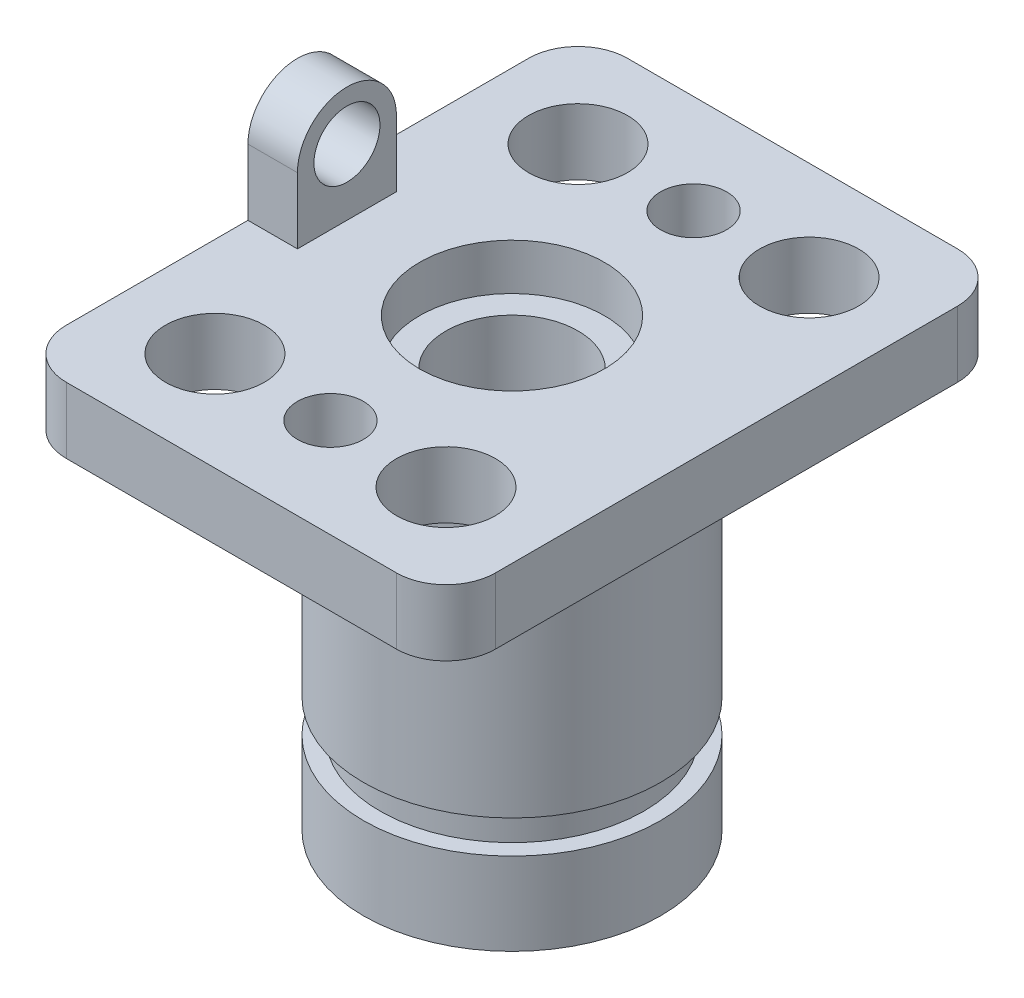
ISO-10303-21;
HEADER;
FILE_DESCRIPTION(('STEP AP214'),'2;1');
FILE_NAME('part.step','',(''),(''),'','','');
FILE_SCHEMA(('AUTOMOTIVE_DESIGN { 1 0 10303 214 1 1 1 1 }'));
ENDSEC;
DATA;
#1=APPLICATION_CONTEXT('core data for automotive mechanical design processes');
#2=APPLICATION_PROTOCOL_DEFINITION('international standard','automotive_design',2000,#1);
#3=PRODUCT_CONTEXT('',#1,'mechanical');
#4=PRODUCT('Part','Part','',(#3));
#5=PRODUCT_RELATED_PRODUCT_CATEGORY('part','',(#4));
#6=PRODUCT_DEFINITION_FORMATION('','',#4);
#7=PRODUCT_DEFINITION_CONTEXT('part definition',#1,'design');
#8=PRODUCT_DEFINITION('design','',#6,#7);
#9=PRODUCT_DEFINITION_SHAPE('','',#8);
#10=(LENGTH_UNIT() NAMED_UNIT(*) SI_UNIT(.MILLI.,.METRE.));
#11=(NAMED_UNIT(*) PLANE_ANGLE_UNIT() SI_UNIT($,.RADIAN.));
#12=(NAMED_UNIT(*) SI_UNIT($,.STERADIAN.) SOLID_ANGLE_UNIT());
#13=UNCERTAINTY_MEASURE_WITH_UNIT(LENGTH_MEASURE(1.E-05),#10,'distance_accuracy_value','');
#14=(GEOMETRIC_REPRESENTATION_CONTEXT(3) GLOBAL_UNCERTAINTY_ASSIGNED_CONTEXT((#13)) GLOBAL_UNIT_ASSIGNED_CONTEXT((#10,
#11,#12)) REPRESENTATION_CONTEXT('',''));
#15=CARTESIAN_POINT('',(0.,0.,0.));
#16=DIRECTION('',(0.,0.,1.));
#17=DIRECTION('',(1.,0.,0.));
#18=AXIS2_PLACEMENT_3D('',#15,#16,#17);
#19=CARTESIAN_POINT('',(0.,135.,0.));
#20=DIRECTION('',(0.,-1.,0.));
#21=DIRECTION('',(0.,0.,-1.));
#22=AXIS2_PLACEMENT_3D('',#19,#20,#21);
#23=PLANE('',#22);
#24=CARTESIAN_POINT('',(35.,135.,-55.));
#25=DIRECTION('',(0.,1.,0.));
#26=DIRECTION('',(0.,0.,1.));
#27=AXIS2_PLACEMENT_3D('',#24,#25,#26);
#28=CIRCLE('',#27,15.);
#29=CARTESIAN_POINT('',(35.,135.,-40.));
#30=VERTEX_POINT('',#29);
#31=EDGE_CURVE('E224',#30,#30,#28,.T.);
#32=ORIENTED_EDGE('',*,*,#31,.F.);
#33=EDGE_LOOP('',(#32));
#34=FACE_BOUND('',#33,.T.);
#35=CARTESIAN_POINT('',(0.,135.,-55.));
#36=DIRECTION('',(0.,1.,0.));
#37=DIRECTION('',(0.,0.,1.));
#38=AXIS2_PLACEMENT_3D('',#35,#36,#37);
#39=CIRCLE('',#38,10.);
#40=CARTESIAN_POINT('',(0.,135.,-45.));
#41=VERTEX_POINT('',#40);
#42=EDGE_CURVE('E226',#41,#41,#39,.T.);
#43=ORIENTED_EDGE('',*,*,#42,.F.);
#44=EDGE_LOOP('',(#43));
#45=FACE_BOUND('',#44,.T.);
#46=CARTESIAN_POINT('',(-35.,135.,-55.));
#47=DIRECTION('',(0.,1.,0.));
#48=DIRECTION('',(0.,0.,1.));
#49=AXIS2_PLACEMENT_3D('',#46,#47,#48);
#50=CIRCLE('',#49,15.);
#51=CARTESIAN_POINT('',(-35.,135.,-40.));
#52=VERTEX_POINT('',#51);
#53=EDGE_CURVE('E247',#52,#52,#50,.T.);
#54=ORIENTED_EDGE('',*,*,#53,.F.);
#55=EDGE_LOOP('',(#54));
#56=FACE_BOUND('',#55,.T.);
#57=CARTESIAN_POINT('',(-35.,135.,55.));
#58=DIRECTION('',(0.,1.,0.));
#59=DIRECTION('',(0.,0.,-1.));
#60=AXIS2_PLACEMENT_3D('',#57,#58,#59);
#61=CIRCLE('',#60,15.);
#62=CARTESIAN_POINT('',(-35.,135.,40.));
#63=VERTEX_POINT('',#62);
#64=EDGE_CURVE('E243',#63,#63,#61,.T.);
#65=ORIENTED_EDGE('',*,*,#64,.F.);
#66=EDGE_LOOP('',(#65));
#67=FACE_BOUND('',#66,.T.);
#68=CARTESIAN_POINT('',(0.,135.,55.));
#69=DIRECTION('',(0.,1.,0.));
#70=DIRECTION('',(0.,0.,-1.));
#71=AXIS2_PLACEMENT_3D('',#68,#69,#70);
#72=CIRCLE('',#71,10.);
#73=CARTESIAN_POINT('',(0.,135.,45.));
#74=VERTEX_POINT('',#73);
#75=EDGE_CURVE('E240',#74,#74,#72,.T.);
#76=ORIENTED_EDGE('',*,*,#75,.F.);
#77=EDGE_LOOP('',(#76));
#78=FACE_BOUND('',#77,.T.);
#79=CARTESIAN_POINT('',(35.,135.,55.));
#80=DIRECTION('',(0.,1.,0.));
#81=DIRECTION('',(0.,0.,-1.));
#82=AXIS2_PLACEMENT_3D('',#79,#80,#81);
#83=CIRCLE('',#82,15.);
#84=CARTESIAN_POINT('',(35.,135.,40.));
#85=VERTEX_POINT('',#84);
#86=EDGE_CURVE('E231',#85,#85,#83,.T.);
#87=ORIENTED_EDGE('',*,*,#86,.F.);
#88=EDGE_LOOP('',(#87));
#89=FACE_BOUND('',#88,.T.);
#90=CARTESIAN_POINT('',(0.,135.,0.));
#91=DIRECTION('',(0.,1.,0.));
#92=DIRECTION('',(0.,0.,1.));
#93=AXIS2_PLACEMENT_3D('',#90,#91,#92);
#94=CIRCLE('',#93,28.);
#95=CARTESIAN_POINT('',(0.,135.,28.));
#96=VERTEX_POINT('',#95);
#97=EDGE_CURVE('E236',#96,#96,#94,.T.);
#98=ORIENTED_EDGE('',*,*,#97,.F.);
#99=EDGE_LOOP('',(#98));
#100=FACE_BOUND('',#99,.T.);
#101=DIRECTION('',(0.,0.,1.));
#102=VECTOR('',#101,1.);
#103=CARTESIAN_POINT('',(-65.,135.,85.));
#104=LINE('',#103,#102);
#105=CARTESIAN_POINT('',(-65.,135.,15.));
#106=VERTEX_POINT('',#105);
#107=CARTESIAN_POINT('',(-65.,135.,70.));
#108=VERTEX_POINT('',#107);
#109=EDGE_CURVE('E223',#106,#108,#104,.T.);
#110=ORIENTED_EDGE('',*,*,#109,.T.);
#111=CARTESIAN_POINT('',(-50.,135.,70.));
#112=DIRECTION('',(0.,-1.,0.));
#113=DIRECTION('',(0.,0.,-1.));
#114=AXIS2_PLACEMENT_3D('',#111,#112,#113);
#115=CIRCLE('',#114,15.);
#116=CARTESIAN_POINT('',(-50.,135.,85.));
#117=VERTEX_POINT('',#116);
#118=EDGE_CURVE('E289',#108,#117,#115,.F.);
#119=ORIENTED_EDGE('',*,*,#118,.T.);
#120=DIRECTION('',(1.,0.,0.));
#121=VECTOR('',#120,1.);
#122=CARTESIAN_POINT('',(-65.,135.,85.));
#123=LINE('',#122,#121);
#124=CARTESIAN_POINT('',(50.,135.,85.));
#125=VERTEX_POINT('',#124);
#126=EDGE_CURVE('E213',#117,#125,#123,.T.);
#127=ORIENTED_EDGE('',*,*,#126,.T.);
#128=CARTESIAN_POINT('',(50.,135.,70.));
#129=DIRECTION('',(0.,-1.,0.));
#130=DIRECTION('',(0.,0.,-1.));
#131=AXIS2_PLACEMENT_3D('',#128,#129,#130);
#132=CIRCLE('',#131,15.);
#133=CARTESIAN_POINT('',(65.,135.,70.));
#134=VERTEX_POINT('',#133);
#135=EDGE_CURVE('E286',#125,#134,#132,.F.);
#136=ORIENTED_EDGE('',*,*,#135,.T.);
#137=DIRECTION('',(0.,0.,-1.));
#138=VECTOR('',#137,1.);
#139=CARTESIAN_POINT('',(65.,135.,85.));
#140=LINE('',#139,#138);
#141=CARTESIAN_POINT('',(65.,135.,-70.));
#142=VERTEX_POINT('',#141);
#143=EDGE_CURVE('E207',#134,#142,#140,.T.);
#144=ORIENTED_EDGE('',*,*,#143,.T.);
#145=CARTESIAN_POINT('',(50.,135.,-70.));
#146=DIRECTION('',(0.,-1.,0.));
#147=DIRECTION('',(0.,0.,-1.));
#148=AXIS2_PLACEMENT_3D('',#145,#146,#147);
#149=CIRCLE('',#148,15.);
#150=CARTESIAN_POINT('',(50.,135.,-85.));
#151=VERTEX_POINT('',#150);
#152=EDGE_CURVE('E56',#142,#151,#149,.F.);
#153=ORIENTED_EDGE('',*,*,#152,.T.);
#154=DIRECTION('',(-1.,0.,0.));
#155=VECTOR('',#154,1.);
#156=CARTESIAN_POINT('',(-65.,135.,-85.));
#157=LINE('',#156,#155);
#158=CARTESIAN_POINT('',(-50.,135.,-85.));
#159=VERTEX_POINT('',#158);
#160=EDGE_CURVE('E225',#151,#159,#157,.T.);
#161=ORIENTED_EDGE('',*,*,#160,.T.);
#162=CARTESIAN_POINT('',(-50.,135.,-70.));
#163=DIRECTION('',(0.,-1.,0.));
#164=DIRECTION('',(0.,0.,-1.));
#165=AXIS2_PLACEMENT_3D('',#162,#163,#164);
#166=CIRCLE('',#165,15.);
#167=CARTESIAN_POINT('',(-65.,135.,-70.));
#168=VERTEX_POINT('',#167);
#169=EDGE_CURVE('E288',#159,#168,#166,.F.);
#170=ORIENTED_EDGE('',*,*,#169,.T.);
#171=CARTESIAN_POINT('',(-65.,135.,-15.));
#172=VERTEX_POINT('',#171);
#173=EDGE_CURVE('E219',#168,#172,#104,.T.);
#174=ORIENTED_EDGE('',*,*,#173,.T.);
#175=DIRECTION('',(-1.,0.,0.));
#176=VECTOR('',#175,1.);
#177=CARTESIAN_POINT('',(-50.,135.,-15.));
#178=LINE('',#177,#176);
#179=CARTESIAN_POINT('',(-50.,135.,-15.));
#180=VERTEX_POINT('',#179);
#181=EDGE_CURVE('E147',#180,#172,#178,.T.);
#182=ORIENTED_EDGE('',*,*,#181,.F.);
#183=DIRECTION('',(0.,0.,1.));
#184=VECTOR('',#183,1.);
#185=CARTESIAN_POINT('',(-50.,135.,-15.));
#186=LINE('',#185,#184);
#187=CARTESIAN_POINT('',(-50.,135.,15.));
#188=VERTEX_POINT('',#187);
#189=EDGE_CURVE('E158',#180,#188,#186,.T.);
#190=ORIENTED_EDGE('',*,*,#189,.T.);
#191=DIRECTION('',(-1.,0.,0.));
#192=VECTOR('',#191,1.);
#193=CARTESIAN_POINT('',(-50.,135.,15.));
#194=LINE('',#193,#192);
#195=EDGE_CURVE('E176',#188,#106,#194,.T.);
#196=ORIENTED_EDGE('',*,*,#195,.T.);
#197=EDGE_LOOP('',(#110,#119,#127,#136,#144,#153,#161,#170,#174,#182,#190,#196));
#198=FACE_BOUND('',#197,.T.);
#199=ADVANCED_FACE('F39',(#34,#45,#56,#67,#78,#89,#100,#198),#23,.F.);
#200=CARTESIAN_POINT('',(0.,115.,0.));
#201=DIRECTION('',(0.,-1.,0.));
#202=DIRECTION('',(0.,0.,-1.));
#203=AXIS2_PLACEMENT_3D('',#200,#201,#202);
#204=CYLINDRICAL_SURFACE('',#203,45.);
#205=CARTESIAN_POINT('',(0.,115.,0.));
#206=DIRECTION('',(0.,1.,0.));
#207=DIRECTION('',(0.,0.,1.));
#208=AXIS2_PLACEMENT_3D('',#205,#206,#207);
#209=CIRCLE('',#208,45.);
#210=CARTESIAN_POINT('',(0.,115.,45.));
#211=VERTEX_POINT('',#210);
#212=CARTESIAN_POINT('',(0.,115.,-45.));
#213=VERTEX_POINT('',#212);
#214=EDGE_CURVE('E200',#211,#213,#209,.T.);
#215=ORIENTED_EDGE('',*,*,#214,.F.);
#216=EDGE_CURVE('E205',#213,#211,#209,.T.);
#217=ORIENTED_EDGE('',*,*,#216,.F.);
#218=EDGE_LOOP('',(#215,#217));
#219=FACE_BOUND('',#218,.T.);
#220=CARTESIAN_POINT('',(0.,35.0000000000001,0.));
#221=DIRECTION('',(0.,-1.,0.));
#222=DIRECTION('',(1.,0.,0.));
#223=AXIS2_PLACEMENT_3D('',#220,#221,#222);
#224=CIRCLE('',#223,45.);
#225=CARTESIAN_POINT('',(45.,35.0000000000001,0.));
#226=VERTEX_POINT('',#225);
#227=EDGE_CURVE('E198',#226,#226,#224,.T.);
#228=ORIENTED_EDGE('',*,*,#227,.F.);
#229=EDGE_LOOP('',(#228));
#230=FACE_BOUND('',#229,.T.);
#231=ADVANCED_FACE('F339',(#219,#230),#204,.T.);
#232=CARTESIAN_POINT('',(0.,0.,0.));
#233=DIRECTION('',(0.,1.,0.));
#234=DIRECTION('',(0.,0.,1.));
#235=AXIS2_PLACEMENT_3D('',#232,#233,#234);
#236=CYLINDRICAL_SURFACE('',#235,20.);
#237=CARTESIAN_POINT('',(0.,121.,0.));
#238=DIRECTION('',(0.,1.,0.));
#239=DIRECTION('',(0.,0.,1.));
#240=AXIS2_PLACEMENT_3D('',#237,#238,#239);
#241=CIRCLE('',#240,20.);
#242=CARTESIAN_POINT('',(0.,121.,20.));
#243=VERTEX_POINT('',#242);
#244=EDGE_CURVE('E192',#243,#243,#241,.T.);
#245=ORIENTED_EDGE('',*,*,#244,.T.);
#246=EDGE_LOOP('',(#245));
#247=FACE_BOUND('',#246,.T.);
#248=CARTESIAN_POINT('',(0.,0.,0.));
#249=DIRECTION('',(0.,1.,0.));
#250=DIRECTION('',(0.,0.,1.));
#251=AXIS2_PLACEMENT_3D('',#248,#249,#250);
#252=CIRCLE('',#251,20.);
#253=CARTESIAN_POINT('',(0.,0.,20.));
#254=VERTEX_POINT('',#253);
#255=EDGE_CURVE('E185',#254,#254,#252,.T.);
#256=ORIENTED_EDGE('',*,*,#255,.F.);
#257=EDGE_LOOP('',(#256));
#258=FACE_BOUND('',#257,.T.);
#259=ADVANCED_FACE('F350',(#247,#258),#236,.F.);
#260=CARTESIAN_POINT('',(65.,135.,85.));
#261=DIRECTION('',(-1.,0.,0.));
#262=DIRECTION('',(0.,0.,1.));
#263=AXIS2_PLACEMENT_3D('',#260,#261,#262);
#264=PLANE('',#263);
#265=ORIENTED_EDGE('',*,*,#143,.F.);
#266=DIRECTION('',(0.,-1.,0.));
#267=VECTOR('',#266,1.);
#268=CARTESIAN_POINT('',(65.,135.,70.));
#269=LINE('',#268,#267);
#270=CARTESIAN_POINT('',(65.,115.,70.));
#271=VERTEX_POINT('',#270);
#272=EDGE_CURVE('E295',#134,#271,#269,.T.);
#273=ORIENTED_EDGE('',*,*,#272,.T.);
#274=DIRECTION('',(0.,0.,-1.));
#275=VECTOR('',#274,1.);
#276=CARTESIAN_POINT('',(65.,115.,85.));
#277=LINE('',#276,#275);
#278=CARTESIAN_POINT('',(65.,115.,-70.));
#279=VERTEX_POINT('',#278);
#280=EDGE_CURVE('E215',#271,#279,#277,.T.);
#281=ORIENTED_EDGE('',*,*,#280,.T.);
#282=DIRECTION('',(0.,-1.,0.));
#283=VECTOR('',#282,1.);
#284=CARTESIAN_POINT('',(65.,135.,-70.));
#285=LINE('',#284,#283);
#286=EDGE_CURVE('E292',#279,#142,#285,.F.);
#287=ORIENTED_EDGE('',*,*,#286,.T.);
#288=EDGE_LOOP('',(#265,#273,#281,#287));
#289=FACE_BOUND('',#288,.T.);
#290=ADVANCED_FACE('F333',(#289),#264,.F.);
#291=CARTESIAN_POINT('',(-65.,135.,-85.));
#292=DIRECTION('',(0.,0.,1.));
#293=DIRECTION('',(1.,0.,0.));
#294=AXIS2_PLACEMENT_3D('',#291,#292,#293);
#295=PLANE('',#294);
#296=DIRECTION('',(-1.,0.,0.));
#297=VECTOR('',#296,1.);
#298=CARTESIAN_POINT('',(-65.,115.,-85.));
#299=LINE('',#298,#297);
#300=CARTESIAN_POINT('',(50.,115.,-85.));
#301=VERTEX_POINT('',#300);
#302=CARTESIAN_POINT('',(-50.,115.,-85.));
#303=VERTEX_POINT('',#302);
#304=EDGE_CURVE('E208',#301,#303,#299,.T.);
#305=ORIENTED_EDGE('',*,*,#304,.T.);
#306=DIRECTION('',(0.,-1.,0.));
#307=VECTOR('',#306,1.);
#308=CARTESIAN_POINT('',(-50.,135.,-85.));
#309=LINE('',#308,#307);
#310=EDGE_CURVE('E11',#303,#159,#309,.F.);
#311=ORIENTED_EDGE('',*,*,#310,.T.);
#312=ORIENTED_EDGE('',*,*,#160,.F.);
#313=DIRECTION('',(0.,-1.,0.));
#314=VECTOR('',#313,1.);
#315=CARTESIAN_POINT('',(50.,135.,-85.));
#316=LINE('',#315,#314);
#317=EDGE_CURVE('E50',#151,#301,#316,.T.);
#318=ORIENTED_EDGE('',*,*,#317,.T.);
#319=EDGE_LOOP('',(#305,#311,#312,#318));
#320=FACE_BOUND('',#319,.T.);
#321=ADVANCED_FACE('F299',(#320),#295,.F.);
#322=CARTESIAN_POINT('',(-65.,135.,85.));
#323=DIRECTION('',(1.,0.,0.));
#324=DIRECTION('',(0.,0.,-1.));
#325=AXIS2_PLACEMENT_3D('',#322,#323,#324);
#326=PLANE('',#325);
#327=CARTESIAN_POINT('',(-65.,155.,0.));
#328=DIRECTION('',(-1.,0.,0.));
#329=DIRECTION('',(0.,0.,1.));
#330=AXIS2_PLACEMENT_3D('',#327,#328,#329);
#331=CIRCLE('',#330,10.);
#332=CARTESIAN_POINT('',(-65.,155.,9.99999999999999));
#333=VERTEX_POINT('',#332);
#334=EDGE_CURVE('E164',#333,#333,#331,.T.);
#335=ORIENTED_EDGE('',*,*,#334,.F.);
#336=EDGE_LOOP('',(#335));
#337=FACE_BOUND('',#336,.T.);
#338=DIRECTION('',(0.,0.,1.));
#339=VECTOR('',#338,1.);
#340=CARTESIAN_POINT('',(-65.,115.,85.));
#341=LINE('',#340,#339);
#342=CARTESIAN_POINT('',(-65.,115.,-70.));
#343=VERTEX_POINT('',#342);
#344=CARTESIAN_POINT('',(-65.,115.,70.));
#345=VERTEX_POINT('',#344);
#346=EDGE_CURVE('E210',#343,#345,#341,.T.);
#347=ORIENTED_EDGE('',*,*,#346,.T.);
#348=DIRECTION('',(0.,-1.,0.));
#349=VECTOR('',#348,1.);
#350=CARTESIAN_POINT('',(-65.,135.,70.));
#351=LINE('',#350,#349);
#352=EDGE_CURVE('E281',#345,#108,#351,.F.);
#353=ORIENTED_EDGE('',*,*,#352,.T.);
#354=ORIENTED_EDGE('',*,*,#109,.F.);
#355=DIRECTION('',(0.,1.,0.));
#356=VECTOR('',#355,1.);
#357=CARTESIAN_POINT('',(-65.,135.,15.));
#358=LINE('',#357,#356);
#359=CARTESIAN_POINT('',(-65.,155.,15.));
#360=VERTEX_POINT('',#359);
#361=EDGE_CURVE('E159',#106,#360,#358,.T.);
#362=ORIENTED_EDGE('',*,*,#361,.T.);
#363=CARTESIAN_POINT('',(-65.,155.,0.));
#364=DIRECTION('',(-1.,0.,0.));
#365=DIRECTION('',(0.,0.,1.));
#366=AXIS2_PLACEMENT_3D('',#363,#364,#365);
#367=CIRCLE('',#366,15.);
#368=CARTESIAN_POINT('',(-65.,155.,-15.));
#369=VERTEX_POINT('',#368);
#370=EDGE_CURVE('E167',#360,#369,#367,.T.);
#371=ORIENTED_EDGE('',*,*,#370,.T.);
#372=DIRECTION('',(0.,-1.,0.));
#373=VECTOR('',#372,1.);
#374=CARTESIAN_POINT('',(-65.,155.,-15.));
#375=LINE('',#374,#373);
#376=EDGE_CURVE('E142',#369,#172,#375,.T.);
#377=ORIENTED_EDGE('',*,*,#376,.T.);
#378=ORIENTED_EDGE('',*,*,#173,.F.);
#379=DIRECTION('',(0.,-1.,0.));
#380=VECTOR('',#379,1.);
#381=CARTESIAN_POINT('',(-65.,135.,-70.));
#382=LINE('',#381,#380);
#383=EDGE_CURVE('E278',#168,#343,#382,.T.);
#384=ORIENTED_EDGE('',*,*,#383,.T.);
#385=EDGE_LOOP('',(#347,#353,#354,#362,#371,#377,#378,#384));
#386=FACE_BOUND('',#385,.T.);
#387=ADVANCED_FACE('F315',(#337,#386),#326,.F.);
#388=CARTESIAN_POINT('',(-65.,135.,85.));
#389=DIRECTION('',(0.,0.,-1.));
#390=DIRECTION('',(-1.,0.,0.));
#391=AXIS2_PLACEMENT_3D('',#388,#389,#390);
#392=PLANE('',#391);
#393=ORIENTED_EDGE('',*,*,#126,.F.);
#394=DIRECTION('',(0.,-1.,0.));
#395=VECTOR('',#394,1.);
#396=CARTESIAN_POINT('',(-50.,135.,85.));
#397=LINE('',#396,#395);
#398=CARTESIAN_POINT('',(-50.,115.,85.));
#399=VERTEX_POINT('',#398);
#400=EDGE_CURVE('E267',#117,#399,#397,.T.);
#401=ORIENTED_EDGE('',*,*,#400,.T.);
#402=DIRECTION('',(1.,0.,0.));
#403=VECTOR('',#402,1.);
#404=CARTESIAN_POINT('',(-65.,115.,85.));
#405=LINE('',#404,#403);
#406=CARTESIAN_POINT('',(50.,115.,85.));
#407=VERTEX_POINT('',#406);
#408=EDGE_CURVE('E201',#399,#407,#405,.T.);
#409=ORIENTED_EDGE('',*,*,#408,.T.);
#410=DIRECTION('',(0.,-1.,0.));
#411=VECTOR('',#410,1.);
#412=CARTESIAN_POINT('',(50.,135.,85.));
#413=LINE('',#412,#411);
#414=EDGE_CURVE('E193',#407,#125,#413,.F.);
#415=ORIENTED_EDGE('',*,*,#414,.T.);
#416=EDGE_LOOP('',(#393,#401,#409,#415));
#417=FACE_BOUND('',#416,.T.);
#418=ADVANCED_FACE('F321',(#417),#392,.F.);
#419=CARTESIAN_POINT('',(0.,115.,0.));
#420=DIRECTION('',(0.,-1.,0.));
#421=DIRECTION('',(0.,0.,-1.));
#422=AXIS2_PLACEMENT_3D('',#419,#420,#421);
#423=PLANE('',#422);
#424=CARTESIAN_POINT('',(35.,115.,55.));
#425=DIRECTION('',(0.,1.,0.));
#426=DIRECTION('',(0.,0.,-1.));
#427=AXIS2_PLACEMENT_3D('',#424,#425,#426);
#428=CIRCLE('',#427,15.);
#429=CARTESIAN_POINT('',(35.,115.,40.));
#430=VERTEX_POINT('',#429);
#431=EDGE_CURVE('E216',#430,#430,#428,.T.);
#432=ORIENTED_EDGE('',*,*,#431,.T.);
#433=EDGE_LOOP('',(#432));
#434=FACE_BOUND('',#433,.T.);
#435=CARTESIAN_POINT('',(-35.,115.,55.));
#436=DIRECTION('',(0.,1.,0.));
#437=DIRECTION('',(0.,0.,-1.));
#438=AXIS2_PLACEMENT_3D('',#435,#436,#437);
#439=CIRCLE('',#438,15.);
#440=CARTESIAN_POINT('',(-35.,115.,40.));
#441=VERTEX_POINT('',#440);
#442=EDGE_CURVE('E239',#441,#441,#439,.T.);
#443=ORIENTED_EDGE('',*,*,#442,.T.);
#444=EDGE_LOOP('',(#443));
#445=FACE_BOUND('',#444,.T.);
#446=CARTESIAN_POINT('',(-35.,115.,-55.));
#447=DIRECTION('',(0.,1.,0.));
#448=DIRECTION('',(0.,0.,1.));
#449=AXIS2_PLACEMENT_3D('',#446,#447,#448);
#450=CIRCLE('',#449,15.);
#451=CARTESIAN_POINT('',(-35.,115.,-40.));
#452=VERTEX_POINT('',#451);
#453=EDGE_CURVE('E235',#452,#452,#450,.T.);
#454=ORIENTED_EDGE('',*,*,#453,.T.);
#455=EDGE_LOOP('',(#454));
#456=FACE_BOUND('',#455,.T.);
#457=CARTESIAN_POINT('',(35.,115.,-55.));
#458=DIRECTION('',(0.,1.,0.));
#459=DIRECTION('',(0.,0.,1.));
#460=AXIS2_PLACEMENT_3D('',#457,#458,#459);
#461=CIRCLE('',#460,15.);
#462=CARTESIAN_POINT('',(35.,115.,-40.));
#463=VERTEX_POINT('',#462);
#464=EDGE_CURVE('E230',#463,#463,#461,.T.);
#465=ORIENTED_EDGE('',*,*,#464,.T.);
#466=EDGE_LOOP('',(#465));
#467=FACE_BOUND('',#466,.T.);
#468=ORIENTED_EDGE('',*,*,#216,.T.);
#469=CARTESIAN_POINT('',(0.,115.,55.));
#470=DIRECTION('',(0.,1.,0.));
#471=DIRECTION('',(0.,0.,-1.));
#472=AXIS2_PLACEMENT_3D('',#469,#470,#471);
#473=CIRCLE('',#472,10.);
#474=EDGE_CURVE('E203',#211,#211,#473,.T.);
#475=ORIENTED_EDGE('',*,*,#474,.T.);
#476=ORIENTED_EDGE('',*,*,#214,.T.);
#477=CARTESIAN_POINT('',(0.,115.,-55.));
#478=DIRECTION('',(0.,1.,0.));
#479=DIRECTION('',(0.,0.,1.));
#480=AXIS2_PLACEMENT_3D('',#477,#478,#479);
#481=CIRCLE('',#480,10.);
#482=EDGE_CURVE('E197',#213,#213,#481,.T.);
#483=ORIENTED_EDGE('',*,*,#482,.T.);
#484=EDGE_LOOP('',(#468,#475,#476,#483));
#485=FACE_BOUND('',#484,.T.);
#486=ORIENTED_EDGE('',*,*,#408,.F.);
#487=CARTESIAN_POINT('',(-50.,115.,70.));
#488=DIRECTION('',(0.,-1.,0.));
#489=DIRECTION('',(0.,0.,-1.));
#490=AXIS2_PLACEMENT_3D('',#487,#488,#489);
#491=CIRCLE('',#490,15.);
#492=EDGE_CURVE('E279',#399,#345,#491,.T.);
#493=ORIENTED_EDGE('',*,*,#492,.T.);
#494=ORIENTED_EDGE('',*,*,#346,.F.);
#495=CARTESIAN_POINT('',(-50.,115.,-70.));
#496=DIRECTION('',(0.,-1.,0.));
#497=DIRECTION('',(0.,0.,-1.));
#498=AXIS2_PLACEMENT_3D('',#495,#496,#497);
#499=CIRCLE('',#498,15.);
#500=EDGE_CURVE('E274',#343,#303,#499,.T.);
#501=ORIENTED_EDGE('',*,*,#500,.T.);
#502=ORIENTED_EDGE('',*,*,#304,.F.);
#503=CARTESIAN_POINT('',(50.,115.,-70.));
#504=DIRECTION('',(0.,-1.,0.));
#505=DIRECTION('',(0.,0.,-1.));
#506=AXIS2_PLACEMENT_3D('',#503,#504,#505);
#507=CIRCLE('',#506,15.);
#508=EDGE_CURVE('E275',#301,#279,#507,.T.);
#509=ORIENTED_EDGE('',*,*,#508,.T.);
#510=ORIENTED_EDGE('',*,*,#280,.F.);
#511=CARTESIAN_POINT('',(50.,115.,70.));
#512=DIRECTION('',(0.,-1.,0.));
#513=DIRECTION('',(0.,0.,-1.));
#514=AXIS2_PLACEMENT_3D('',#511,#512,#513);
#515=CIRCLE('',#514,15.);
#516=EDGE_CURVE('E277',#271,#407,#515,.T.);
#517=ORIENTED_EDGE('',*,*,#516,.T.);
#518=EDGE_LOOP('',(#486,#493,#494,#501,#502,#509,#510,#517));
#519=FACE_BOUND('',#518,.T.);
#520=ADVANCED_FACE('F303',(#434,#445,#456,#467,#485,#519),#423,.T.);
#521=CARTESIAN_POINT('',(35.,115.,-55.));
#522=DIRECTION('',(0.,1.,0.));
#523=DIRECTION('',(0.,0.,1.));
#524=AXIS2_PLACEMENT_3D('',#521,#522,#523);
#525=CYLINDRICAL_SURFACE('',#524,15.);
#526=ORIENTED_EDGE('',*,*,#464,.F.);
#527=EDGE_LOOP('',(#526));
#528=FACE_BOUND('',#527,.T.);
#529=ORIENTED_EDGE('',*,*,#31,.T.);
#530=EDGE_LOOP('',(#529));
#531=FACE_BOUND('',#530,.T.);
#532=ADVANCED_FACE('F354',(#528,#531),#525,.F.);
#533=CARTESIAN_POINT('',(0.,115.,-55.));
#534=DIRECTION('',(0.,1.,0.));
#535=DIRECTION('',(0.,0.,1.));
#536=AXIS2_PLACEMENT_3D('',#533,#534,#535);
#537=CYLINDRICAL_SURFACE('',#536,10.);
#538=ORIENTED_EDGE('',*,*,#482,.F.);
#539=EDGE_LOOP('',(#538));
#540=FACE_BOUND('',#539,.T.);
#541=ORIENTED_EDGE('',*,*,#42,.T.);
#542=EDGE_LOOP('',(#541));
#543=FACE_BOUND('',#542,.T.);
#544=ADVANCED_FACE('F356',(#540,#543),#537,.F.);
#545=CARTESIAN_POINT('',(-35.,115.,-55.));
#546=DIRECTION('',(0.,1.,0.));
#547=DIRECTION('',(0.,0.,1.));
#548=AXIS2_PLACEMENT_3D('',#545,#546,#547);
#549=CYLINDRICAL_SURFACE('',#548,15.);
#550=ORIENTED_EDGE('',*,*,#453,.F.);
#551=EDGE_LOOP('',(#550));
#552=FACE_BOUND('',#551,.T.);
#553=ORIENTED_EDGE('',*,*,#53,.T.);
#554=EDGE_LOOP('',(#553));
#555=FACE_BOUND('',#554,.T.);
#556=ADVANCED_FACE('F375',(#552,#555),#549,.F.);
#557=CARTESIAN_POINT('',(-35.,115.,55.));
#558=DIRECTION('',(0.,1.,0.));
#559=DIRECTION('',(0.,0.,1.));
#560=AXIS2_PLACEMENT_3D('',#557,#558,#559);
#561=CYLINDRICAL_SURFACE('',#560,15.);
#562=ORIENTED_EDGE('',*,*,#442,.F.);
#563=EDGE_LOOP('',(#562));
#564=FACE_BOUND('',#563,.T.);
#565=ORIENTED_EDGE('',*,*,#64,.T.);
#566=EDGE_LOOP('',(#565));
#567=FACE_BOUND('',#566,.T.);
#568=ADVANCED_FACE('F368',(#564,#567),#561,.F.);
#569=CARTESIAN_POINT('',(0.,115.,55.));
#570=DIRECTION('',(0.,1.,0.));
#571=DIRECTION('',(0.,0.,1.));
#572=AXIS2_PLACEMENT_3D('',#569,#570,#571);
#573=CYLINDRICAL_SURFACE('',#572,10.);
#574=ORIENTED_EDGE('',*,*,#474,.F.);
#575=EDGE_LOOP('',(#574));
#576=FACE_BOUND('',#575,.T.);
#577=ORIENTED_EDGE('',*,*,#75,.T.);
#578=EDGE_LOOP('',(#577));
#579=FACE_BOUND('',#578,.T.);
#580=ADVANCED_FACE('F364',(#576,#579),#573,.F.);
#581=CARTESIAN_POINT('',(35.,115.,55.));
#582=DIRECTION('',(0.,1.,0.));
#583=DIRECTION('',(0.,0.,1.));
#584=AXIS2_PLACEMENT_3D('',#581,#582,#583);
#585=CYLINDRICAL_SURFACE('',#584,15.);
#586=ORIENTED_EDGE('',*,*,#431,.F.);
#587=EDGE_LOOP('',(#586));
#588=FACE_BOUND('',#587,.T.);
#589=ORIENTED_EDGE('',*,*,#86,.T.);
#590=EDGE_LOOP('',(#589));
#591=FACE_BOUND('',#590,.T.);
#592=ADVANCED_FACE('F359',(#588,#591),#585,.F.);
#593=CARTESIAN_POINT('',(0.,121.,0.));
#594=DIRECTION('',(0.,1.,0.));
#595=DIRECTION('',(0.,0.,1.));
#596=AXIS2_PLACEMENT_3D('',#593,#594,#595);
#597=CYLINDRICAL_SURFACE('',#596,28.);
#598=CARTESIAN_POINT('',(0.,121.,0.));
#599=DIRECTION('',(0.,1.,0.));
#600=DIRECTION('',(0.,0.,1.));
#601=AXIS2_PLACEMENT_3D('',#598,#599,#600);
#602=CIRCLE('',#601,28.);
#603=CARTESIAN_POINT('',(0.,121.,28.));
#604=VERTEX_POINT('',#603);
#605=EDGE_CURVE('E263',#604,#604,#602,.T.);
#606=ORIENTED_EDGE('',*,*,#605,.F.);
#607=EDGE_LOOP('',(#606));
#608=FACE_BOUND('',#607,.T.);
#609=ORIENTED_EDGE('',*,*,#97,.T.);
#610=EDGE_LOOP('',(#609));
#611=FACE_BOUND('',#610,.T.);
#612=ADVANCED_FACE('F361',(#608,#611),#597,.F.);
#613=CARTESIAN_POINT('',(0.,121.,0.));
#614=DIRECTION('',(0.,1.,0.));
#615=DIRECTION('',(0.,0.,1.));
#616=AXIS2_PLACEMENT_3D('',#613,#614,#615);
#617=PLANE('',#616);
#618=ORIENTED_EDGE('',*,*,#244,.F.);
#619=EDGE_LOOP('',(#618));
#620=FACE_BOUND('',#619,.T.);
#621=ORIENTED_EDGE('',*,*,#605,.T.);
#622=EDGE_LOOP('',(#621));
#623=FACE_BOUND('',#622,.T.);
#624=ADVANCED_FACE('F385',(#620,#623),#617,.T.);
#625=CARTESIAN_POINT('',(-45.,35.,0.));
#626=DIRECTION('',(0.,-1.,0.));
#627=DIRECTION('',(1.,0.,0.));
#628=AXIS2_PLACEMENT_3D('',#625,#626,#627);
#629=PLANE('',#628);
#630=CARTESIAN_POINT('',(0.,35.0000000000002,0.));
#631=DIRECTION('',(0.,-1.,0.));
#632=DIRECTION('',(1.,0.,0.));
#633=AXIS2_PLACEMENT_3D('',#630,#631,#632);
#634=CIRCLE('',#633,40.);
#635=CARTESIAN_POINT('',(40.,35.0000000000004,0.));
#636=VERTEX_POINT('',#635);
#637=EDGE_CURVE('E195',#636,#636,#634,.T.);
#638=ORIENTED_EDGE('',*,*,#637,.F.);
#639=EDGE_LOOP('',(#638));
#640=FACE_BOUND('',#639,.T.);
#641=ORIENTED_EDGE('',*,*,#227,.T.);
#642=EDGE_LOOP('',(#641));
#643=FACE_BOUND('',#642,.T.);
#644=ADVANCED_FACE('F387',(#640,#643),#629,.T.);
#645=CARTESIAN_POINT('',(0.,25.0000000000001,0.));
#646=DIRECTION('',(0.,-1.,0.));
#647=DIRECTION('',(1.,0.,0.));
#648=AXIS2_PLACEMENT_3D('',#645,#646,#647);
#649=CYLINDRICAL_SURFACE('',#648,40.);
#650=CARTESIAN_POINT('',(0.,25.0000000000002,0.));
#651=DIRECTION('',(0.,-1.,0.));
#652=DIRECTION('',(1.,0.,0.));
#653=AXIS2_PLACEMENT_3D('',#650,#651,#652);
#654=CIRCLE('',#653,40.);
#655=CARTESIAN_POINT('',(40.0000000000001,25.0000000000004,0.));
#656=VERTEX_POINT('',#655);
#657=EDGE_CURVE('E189',#656,#656,#654,.T.);
#658=ORIENTED_EDGE('',*,*,#657,.F.);
#659=EDGE_LOOP('',(#658));
#660=FACE_BOUND('',#659,.T.);
#661=ORIENTED_EDGE('',*,*,#637,.T.);
#662=EDGE_LOOP('',(#661));
#663=FACE_BOUND('',#662,.T.);
#664=ADVANCED_FACE('F386',(#660,#663),#649,.T.);
#665=CARTESIAN_POINT('',(0.,115.,0.));
#666=DIRECTION('',(0.,-1.,0.));
#667=DIRECTION('',(0.,0.,-1.));
#668=AXIS2_PLACEMENT_3D('',#665,#666,#667);
#669=CYLINDRICAL_SURFACE('',#668,45.);
#670=CARTESIAN_POINT('',(0.,0.,0.));
#671=DIRECTION('',(0.,1.,0.));
#672=DIRECTION('',(0.,0.,1.));
#673=AXIS2_PLACEMENT_3D('',#670,#671,#672);
#674=CIRCLE('',#673,45.);
#675=CARTESIAN_POINT('',(0.,0.,45.));
#676=VERTEX_POINT('',#675);
#677=EDGE_CURVE('E184',#676,#676,#674,.T.);
#678=ORIENTED_EDGE('',*,*,#677,.T.);
#679=EDGE_LOOP('',(#678));
#680=FACE_BOUND('',#679,.T.);
#681=CARTESIAN_POINT('',(0.,25.0000000000001,0.));
#682=DIRECTION('',(0.,-1.,0.));
#683=DIRECTION('',(1.,0.,0.));
#684=AXIS2_PLACEMENT_3D('',#681,#682,#683);
#685=CIRCLE('',#684,45.);
#686=CARTESIAN_POINT('',(45.,25.0000000000001,0.));
#687=VERTEX_POINT('',#686);
#688=EDGE_CURVE('E174',#687,#687,#685,.T.);
#689=ORIENTED_EDGE('',*,*,#688,.T.);
#690=EDGE_LOOP('',(#689));
#691=FACE_BOUND('',#690,.T.);
#692=ADVANCED_FACE('F508',(#680,#691),#669,.T.);
#693=CARTESIAN_POINT('',(0.,0.,0.));
#694=DIRECTION('',(0.,1.,0.));
#695=DIRECTION('',(0.,0.,1.));
#696=AXIS2_PLACEMENT_3D('',#693,#694,#695);
#697=PLANE('',#696);
#698=ORIENTED_EDGE('',*,*,#255,.T.);
#699=EDGE_LOOP('',(#698));
#700=FACE_BOUND('',#699,.T.);
#701=ORIENTED_EDGE('',*,*,#677,.F.);
#702=EDGE_LOOP('',(#701));
#703=FACE_BOUND('',#702,.T.);
#704=ADVANCED_FACE('F514',(#700,#703),#697,.F.);
#705=CARTESIAN_POINT('',(0.,25.,0.));
#706=DIRECTION('',(0.,1.,0.));
#707=DIRECTION('',(-1.,0.,0.));
#708=AXIS2_PLACEMENT_3D('',#705,#706,#707);
#709=PLANE('',#708);
#710=ORIENTED_EDGE('',*,*,#657,.T.);
#711=EDGE_LOOP('',(#710));
#712=FACE_BOUND('',#711,.T.);
#713=ORIENTED_EDGE('',*,*,#688,.F.);
#714=EDGE_LOOP('',(#713));
#715=FACE_BOUND('',#714,.T.);
#716=ADVANCED_FACE('F525',(#712,#715),#709,.T.);
#717=CARTESIAN_POINT('',(-50.,155.,0.));
#718=DIRECTION('',(-1.,0.,0.));
#719=DIRECTION('',(0.,0.,1.));
#720=AXIS2_PLACEMENT_3D('',#717,#718,#719);
#721=CYLINDRICAL_SURFACE('',#720,15.);
#722=ORIENTED_EDGE('',*,*,#370,.F.);
#723=DIRECTION('',(-1.,0.,0.));
#724=VECTOR('',#723,1.);
#725=CARTESIAN_POINT('',(-50.,155.,15.));
#726=LINE('',#725,#724);
#727=CARTESIAN_POINT('',(-50.,155.,15.));
#728=VERTEX_POINT('',#727);
#729=EDGE_CURVE('E157',#728,#360,#726,.T.);
#730=ORIENTED_EDGE('',*,*,#729,.F.);
#731=CARTESIAN_POINT('',(-50.,155.,0.));
#732=DIRECTION('',(-1.,0.,0.));
#733=DIRECTION('',(0.,0.,1.));
#734=AXIS2_PLACEMENT_3D('',#731,#732,#733);
#735=CIRCLE('',#734,15.);
#736=CARTESIAN_POINT('',(-50.,155.,-15.));
#737=VERTEX_POINT('',#736);
#738=EDGE_CURVE('E151',#728,#737,#735,.T.);
#739=ORIENTED_EDGE('',*,*,#738,.T.);
#740=DIRECTION('',(-1.,0.,0.));
#741=VECTOR('',#740,1.);
#742=CARTESIAN_POINT('',(-50.,155.,-15.));
#743=LINE('',#742,#741);
#744=EDGE_CURVE('E134',#737,#369,#743,.T.);
#745=ORIENTED_EDGE('',*,*,#744,.T.);
#746=EDGE_LOOP('',(#722,#730,#739,#745));
#747=FACE_BOUND('',#746,.T.);
#748=ADVANCED_FACE('F156',(#747),#721,.T.);
#749=CARTESIAN_POINT('',(-50.,135.,15.));
#750=DIRECTION('',(0.,0.,1.));
#751=DIRECTION('',(0.,-1.,0.));
#752=AXIS2_PLACEMENT_3D('',#749,#750,#751);
#753=PLANE('',#752);
#754=ORIENTED_EDGE('',*,*,#361,.F.);
#755=ORIENTED_EDGE('',*,*,#195,.F.);
#756=DIRECTION('',(0.,1.,0.));
#757=VECTOR('',#756,1.);
#758=CARTESIAN_POINT('',(-50.,135.,15.));
#759=LINE('',#758,#757);
#760=EDGE_CURVE('E150',#188,#728,#759,.T.);
#761=ORIENTED_EDGE('',*,*,#760,.T.);
#762=ORIENTED_EDGE('',*,*,#729,.T.);
#763=EDGE_LOOP('',(#754,#755,#761,#762));
#764=FACE_BOUND('',#763,.T.);
#765=ADVANCED_FACE('F551',(#764),#753,.T.);
#766=CARTESIAN_POINT('',(-50.,155.,-15.));
#767=DIRECTION('',(0.,0.,-1.));
#768=DIRECTION('',(0.,1.,0.));
#769=AXIS2_PLACEMENT_3D('',#766,#767,#768);
#770=PLANE('',#769);
#771=ORIENTED_EDGE('',*,*,#376,.F.);
#772=ORIENTED_EDGE('',*,*,#744,.F.);
#773=DIRECTION('',(0.,-1.,0.));
#774=VECTOR('',#773,1.);
#775=CARTESIAN_POINT('',(-50.,155.,-15.));
#776=LINE('',#775,#774);
#777=EDGE_CURVE('E136',#737,#180,#776,.T.);
#778=ORIENTED_EDGE('',*,*,#777,.T.);
#779=ORIENTED_EDGE('',*,*,#181,.T.);
#780=EDGE_LOOP('',(#771,#772,#778,#779));
#781=FACE_BOUND('',#780,.T.);
#782=ADVANCED_FACE('F138',(#781),#770,.T.);
#783=CARTESIAN_POINT('',(-50.,155.,0.));
#784=DIRECTION('',(-1.,0.,0.));
#785=DIRECTION('',(0.,0.,1.));
#786=AXIS2_PLACEMENT_3D('',#783,#784,#785);
#787=PLANE('',#786);
#788=CARTESIAN_POINT('',(-50.,155.,0.));
#789=DIRECTION('',(-1.,0.,0.));
#790=DIRECTION('',(0.,0.,1.));
#791=AXIS2_PLACEMENT_3D('',#788,#789,#790);
#792=CIRCLE('',#791,10.);
#793=CARTESIAN_POINT('',(-50.,155.,9.99999999999999));
#794=VERTEX_POINT('',#793);
#795=EDGE_CURVE('E175',#794,#794,#792,.T.);
#796=ORIENTED_EDGE('',*,*,#795,.T.);
#797=EDGE_LOOP('',(#796));
#798=FACE_BOUND('',#797,.T.);
#799=ORIENTED_EDGE('',*,*,#738,.F.);
#800=ORIENTED_EDGE('',*,*,#760,.F.);
#801=ORIENTED_EDGE('',*,*,#189,.F.);
#802=ORIENTED_EDGE('',*,*,#777,.F.);
#803=EDGE_LOOP('',(#799,#800,#801,#802));
#804=FACE_BOUND('',#803,.T.);
#805=ADVANCED_FACE('F153',(#798,#804),#787,.F.);
#806=CARTESIAN_POINT('',(-50.,155.,0.));
#807=DIRECTION('',(-1.,0.,0.));
#808=DIRECTION('',(0.,0.,1.));
#809=AXIS2_PLACEMENT_3D('',#806,#807,#808);
#810=CYLINDRICAL_SURFACE('',#809,10.);
#811=ORIENTED_EDGE('',*,*,#795,.F.);
#812=EDGE_LOOP('',(#811));
#813=FACE_BOUND('',#812,.T.);
#814=ORIENTED_EDGE('',*,*,#334,.T.);
#815=EDGE_LOOP('',(#814));
#816=FACE_BOUND('',#815,.T.);
#817=ADVANCED_FACE('F398',(#813,#816),#810,.F.);
#818=CARTESIAN_POINT('',(-50.,135.,70.));
#819=DIRECTION('',(0.,-1.,0.));
#820=DIRECTION('',(0.,0.,-1.));
#821=AXIS2_PLACEMENT_3D('',#818,#819,#820);
#822=CYLINDRICAL_SURFACE('',#821,15.);
#823=ORIENTED_EDGE('',*,*,#118,.F.);
#824=ORIENTED_EDGE('',*,*,#352,.F.);
#825=ORIENTED_EDGE('',*,*,#492,.F.);
#826=ORIENTED_EDGE('',*,*,#400,.F.);
#827=EDGE_LOOP('',(#823,#824,#825,#826));
#828=FACE_BOUND('',#827,.T.);
#829=ADVANCED_FACE('F316',(#828),#822,.T.);
#830=CARTESIAN_POINT('',(50.,135.,70.));
#831=DIRECTION('',(0.,-1.,0.));
#832=DIRECTION('',(0.,0.,-1.));
#833=AXIS2_PLACEMENT_3D('',#830,#831,#832);
#834=CYLINDRICAL_SURFACE('',#833,15.);
#835=ORIENTED_EDGE('',*,*,#135,.F.);
#836=ORIENTED_EDGE('',*,*,#414,.F.);
#837=ORIENTED_EDGE('',*,*,#516,.F.);
#838=ORIENTED_EDGE('',*,*,#272,.F.);
#839=EDGE_LOOP('',(#835,#836,#837,#838));
#840=FACE_BOUND('',#839,.T.);
#841=ADVANCED_FACE('F330',(#840),#834,.T.);
#842=CARTESIAN_POINT('',(-50.,135.,-70.));
#843=DIRECTION('',(0.,-1.,0.));
#844=DIRECTION('',(0.,0.,-1.));
#845=AXIS2_PLACEMENT_3D('',#842,#843,#844);
#846=CYLINDRICAL_SURFACE('',#845,15.);
#847=ORIENTED_EDGE('',*,*,#169,.F.);
#848=ORIENTED_EDGE('',*,*,#310,.F.);
#849=ORIENTED_EDGE('',*,*,#500,.F.);
#850=ORIENTED_EDGE('',*,*,#383,.F.);
#851=EDGE_LOOP('',(#847,#848,#849,#850));
#852=FACE_BOUND('',#851,.T.);
#853=ADVANCED_FACE('F307',(#852),#846,.T.);
#854=CARTESIAN_POINT('',(50.,135.,-70.));
#855=DIRECTION('',(0.,-1.,0.));
#856=DIRECTION('',(0.,0.,-1.));
#857=AXIS2_PLACEMENT_3D('',#854,#855,#856);
#858=CYLINDRICAL_SURFACE('',#857,15.);
#859=ORIENTED_EDGE('',*,*,#152,.F.);
#860=ORIENTED_EDGE('',*,*,#286,.F.);
#861=ORIENTED_EDGE('',*,*,#508,.F.);
#862=ORIENTED_EDGE('',*,*,#317,.F.);
#863=EDGE_LOOP('',(#859,#860,#861,#862));
#864=FACE_BOUND('',#863,.T.);
#865=ADVANCED_FACE('F41',(#864),#858,.T.);
#866=CLOSED_SHELL('',(#199,#231,#259,#290,#321,#387,#418,#520,#532,#544,#556,#568,#580,#592,
#612,#624,#644,#664,#692,#704,#716,#748,#765,#782,#805,#817,#829,#841,#853,#865));
#867=MANIFOLD_SOLID_BREP('B2',#866);
#868=ADVANCED_BREP_SHAPE_REPRESENTATION('',(#18,#867),#14);
#869=SHAPE_DEFINITION_REPRESENTATION(#9,#868);
ENDSEC;
END-ISO-10303-21;
